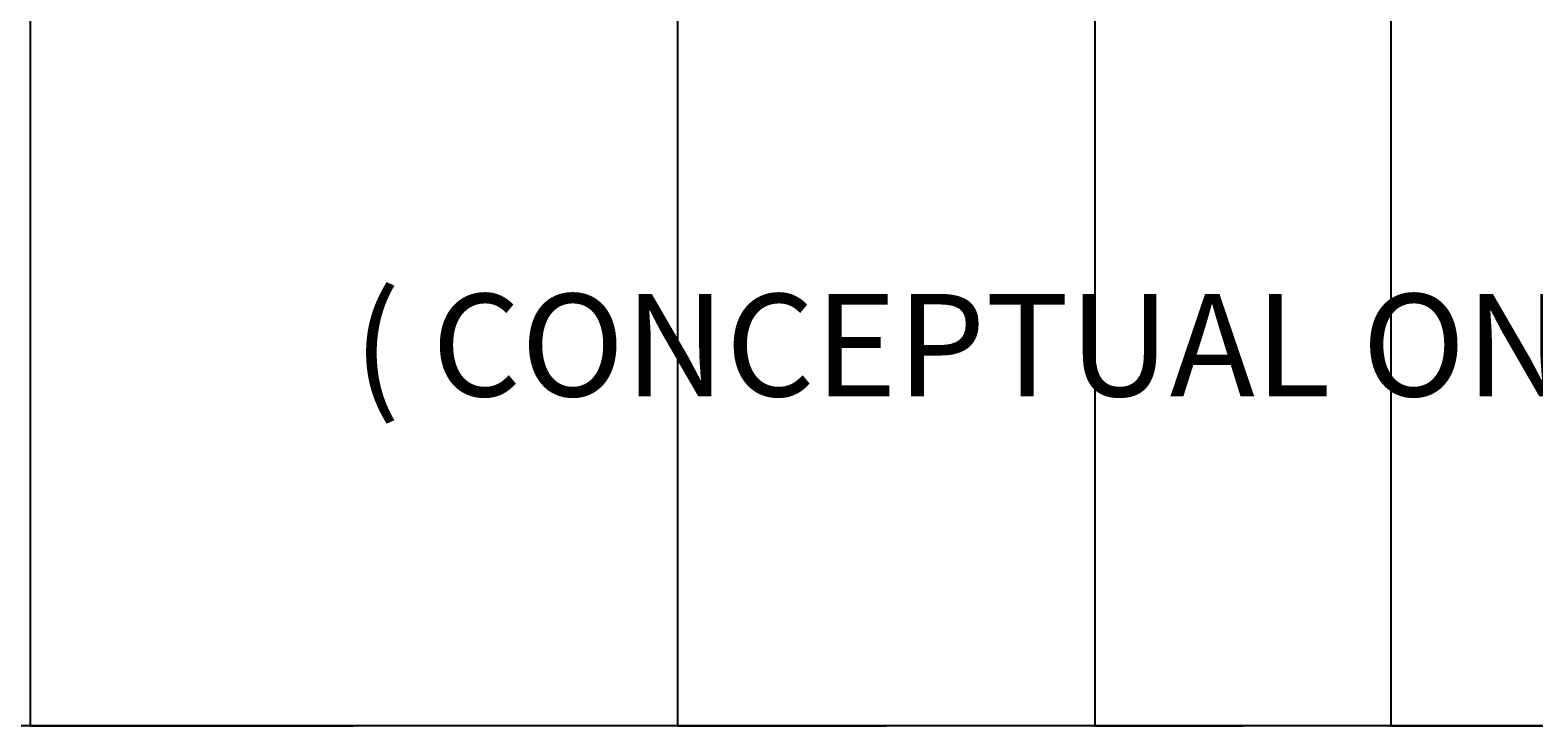
# Model space of a CAD drawing. Units: inches. Extents: x -32109 to 33221, y -19197 to 7608.
# Tile 4 of 25: x -6953 to -741, y -19197 to -16323. Entities that reach past the tile are written whole.
import ezdxf

# ---------------------------------------------------------------- set-up
doc = ezdxf.new("R2010")
doc.units = ezdxf.units.IN
doc.header["$MEASUREMENT"] = 0
doc.layers.add('A-ANNO-DIMS', color=2, linetype='Continuous', lineweight=18)
doc.layers.add('A-ANNO-TEXT', color=7, linetype='Continuous', lineweight=25)
doc.styles.get("Standard").update_dxf_attribs({"font": 'arial.ttf'})
doc.dimstyles.get("Standard").update_dxf_attribs({"dimtxt": 0.18, "dimasz": 0.18, "dimexe": 0.18, "dimexo": 0.0625, "dimgap": 0.09, "dimtad": 0, "dimtih": 1, "dimtoh": 1, "dimdec": 4, "dimzin": 0, "dimdsep": 46, "dimtxsty": 'Standard', "dimcen": 0.09, "dimadec": 0, "dimazin": 0, "dimtfac": 1, "dimtdec": 4, "dimtofl": 0, "dimtmove": 0, "dimatfit": 3, "dimfxl": 1, "dimtolj": 1, "dimtzin": 0, "dimarcsym": 0})

# ---------------------------------------------------------------- blocks, each defined once
blk = doc.blocks.new('*D13')
at = {"layer": 'A-ANNO-DIMS', "color": 0, "lineweight": -2, "transparency": 16777216}
for p, q in [((-21916.3, -16214.9), (-21916.3, -19197.3)), ((5067.2, -16244.2), (5067.2, -19197.3)), ((-21916.1, -19197.2), (-8425, -19197.2)), ((5067, -19197.2), (-8424.2, -19197.2))]:
    blk.add_line(p, q, dxfattribs=at)
at = {"layer": 'A-ANNO-DIMS', "color": 0, "transparency": 16777216}
for points in [[(-21916.1, -19197.1), (-21916.1, -19197.2), (-21916.3, -19197.2)], [(5067, -19197.1), (5067, -19197.2), (5067.2, -19197.2)]]:
    blk.add_solid(points, dxfattribs=at)
at = {"layer": 'Defpoints', "color": 0, "transparency": 16777216}
for p in [(-21916.3, -16214.8), (5067.2, -16244.1), (5067.2, -19197.2)]:
    blk.add_point(p, dxfattribs=at)
at = {"layer": 'A-ANNO-DIMS', "color": 0, "transparency": 16777216, "insert": (-8424.6, -19197.2), "char_height": 0.18, "attachment_point": 5}
blk.add_mtext('\\A1;26983', dxfattribs=at)
blk = doc.blocks.new('*D15')
at = {"layer": 'A-ANNO-DIMS', "color": 0, "lineweight": -2, "transparency": 16777216}
for p, q in [((-8664.1, -16214.9), (-8664.1, -19197.3)), ((-6952.8, -16214.9), (-6952.8, -19197.3)), ((-8664, -19197.2), (-7808.9, -19197.2)), ((-6953, -19197.2), (-7808, -19197.2))]:
    blk.add_line(p, q, dxfattribs=at)
at = {"layer": 'A-ANNO-DIMS', "color": 0, "transparency": 16777216}
for points in [[(-8664, -19197.1), (-8664, -19197.2), (-8664.1, -19197.2)], [(-6953, -19197.1), (-6953, -19197.2), (-6952.8, -19197.2)]]:
    blk.add_solid(points, dxfattribs=at)
at = {"layer": 'Defpoints', "color": 0, "transparency": 16777216}
for p in [(-8664.1, -16214.8), (-6952.8, -16214.8), (-6952.8, -19197.2)]:
    blk.add_point(p, dxfattribs=at)
at = {"layer": 'A-ANNO-DIMS', "color": 0, "transparency": 16777216, "insert": (-7808.5, -19197.2), "char_height": 0.18, "attachment_point": 5}
blk.add_mtext('\\A1;1711.4', dxfattribs=at)
blk = doc.blocks.new('*D103')
at = {"layer": 'A-ANNO-DIMS', "color": 0, "lineweight": -2, "transparency": 16777216}
for p, q in [((-6952.8, -16214.9), (-6952.8, -19197.3)), ((-4279, -16214.9), (-4279, -19197.3)), ((-6952.6, -19197.2), (-5616.2, -19197.2)), ((-4279.1, -19197.2), (-5615.5, -19197.2))]:
    blk.add_line(p, q, dxfattribs=at)
at = {"layer": 'A-ANNO-DIMS', "color": 0, "transparency": 16777216}
for points in [[(-6952.6, -19197.1), (-6952.6, -19197.2), (-6952.8, -19197.2)], [(-4279.1, -19197.1), (-4279.1, -19197.2), (-4279, -19197.2)]]:
    blk.add_solid(points, dxfattribs=at)
at = {"layer": 'Defpoints', "color": 0, "transparency": 16777216}
for p in [(-6952.8, -16214.8), (-4279, -16214.8), (-4279, -19197.2)]:
    blk.add_point(p, dxfattribs=at)
at = {"layer": 'A-ANNO-DIMS', "color": 0, "transparency": 16777216, "insert": (-5615.9, -19197.2), "char_height": 0.18, "attachment_point": 5}
blk.add_mtext('\\A1;2674', dxfattribs=at)
blk = doc.blocks.new('*D104')
at = {"layer": 'A-ANNO-DIMS', "color": 0, "lineweight": -2, "transparency": 16777216}
for p, q in [((-4279, -16214.9), (-4279, -19197.3)), ((-2554.3, -16214.9), (-2554.3, -19197.3)), ((-4278.8, -19197.2), (-3417.1, -19197.2)), ((-2554.5, -19197.2), (-3416.2, -19197.2))]:
    blk.add_line(p, q, dxfattribs=at)
at = {"layer": 'A-ANNO-DIMS', "color": 0, "transparency": 16777216}
for points in [[(-4278.8, -19197.1), (-4278.8, -19197.2), (-4279, -19197.2)], [(-2554.5, -19197.1), (-2554.5, -19197.2), (-2554.3, -19197.2)]]:
    blk.add_solid(points, dxfattribs=at)
at = {"layer": 'Defpoints', "color": 0, "transparency": 16777216}
for p in [(-4279, -16214.8), (-2554.3, -16214.8), (-2554.3, -19197.2)]:
    blk.add_point(p, dxfattribs=at)
at = {"layer": 'A-ANNO-DIMS', "color": 0, "transparency": 16777216, "insert": (-3416.6, -19197.2), "char_height": 0.18, "attachment_point": 5}
blk.add_mtext('\\A1;1724.6', dxfattribs=at)
blk = doc.blocks.new('*D105')
at = {"layer": 'A-ANNO-DIMS', "color": 0, "lineweight": -2, "transparency": 16777216}
for p, q in [((-2554.3, -16214.9), (-2554.3, -19197.3)), ((-1331.3, -16214.9), (-1331.3, -19197.3)), ((-2554.1, -19197.2), (-1943.2, -19197.2)), ((-1331.5, -19197.2), (-1942.5, -19197.2))]:
    blk.add_line(p, q, dxfattribs=at)
at = {"layer": 'A-ANNO-DIMS', "color": 0, "transparency": 16777216}
for points in [[(-2554.1, -19197.1), (-2554.1, -19197.2), (-2554.3, -19197.2)], [(-1331.5, -19197.1), (-1331.5, -19197.2), (-1331.3, -19197.2)]]:
    blk.add_solid(points, dxfattribs=at)
at = {"layer": 'Defpoints', "color": 0, "transparency": 16777216}
for p in [(-2554.3, -16214.8), (-1331.3, -16214.8), (-1331.3, -19197.2)]:
    blk.add_point(p, dxfattribs=at)
at = {"layer": 'A-ANNO-DIMS', "color": 0, "transparency": 16777216, "insert": (-1942.8, -19197.2), "char_height": 0.18, "attachment_point": 5}
blk.add_mtext('\\A1;1223', dxfattribs=at)
blk = doc.blocks.new('*D106')
at = {"layer": 'A-ANNO-DIMS', "color": 0, "lineweight": -2, "transparency": 16777216}
for p, q in [((-1331.3, -16214.9), (-1331.3, -19197.3)), ((2144.2, -16214.9), (2144.2, -19197.3)), ((-1331.1, -19197.2), (406, -19197.2)), ((2144.1, -19197.2), (406.9, -19197.2))]:
    blk.add_line(p, q, dxfattribs=at)
at = {"layer": 'A-ANNO-DIMS', "color": 0, "transparency": 16777216}
for points in [[(-1331.1, -19197.1), (-1331.1, -19197.2), (-1331.3, -19197.2)], [(2144.1, -19197.1), (2144.1, -19197.2), (2144.2, -19197.2)]]:
    blk.add_solid(points, dxfattribs=at)
at = {"layer": 'Defpoints', "color": 0, "transparency": 16777216}
for p in [(-1331.3, -16214.8), (2144.2, -16214.8), (2144.2, -19197.2)]:
    blk.add_point(p, dxfattribs=at)
at = {"layer": 'A-ANNO-DIMS', "color": 0, "transparency": 16777216, "insert": (406.5, -19197.2), "char_height": 0.18, "attachment_point": 5}
blk.add_mtext('\\A1;3475.6', dxfattribs=at)

msp = doc.modelspace()

# ---------------------------------------------------------------- texts
at = {"layer": 'A-ANNO-TEXT'}
msp.add_text('  ( CONCEPTUAL ONLY   NO DIMENSIONS )', height=423.03854, dxfattribs=at).set_placement((-5876.467, -17835.723))

# ---------------------------------------------------------------- dimensions: what is measured, and where the dimension line sits
at = {"layer": 'A-ANNO-DIMS'}
for base, p1, p2, override, picture, middle in [((5067.151, -19197.169), (-21916.328, -16214.811), (5067.151, -16244.113), {"dimdec": 0, "dimlfac": 1, "dimrnd": 0, "dimzin": 0, "dimdsep": 46, "dimlunit": 2}, '*D13', (-8424.588, -19197.169)), ((-6952.774, -19197.169), (-8664.143, -16214.811), (-6952.774, -16214.811), {"dimdec": 1, "dimlfac": 1, "dimrnd": 0, "dimzin": 0, "dimdsep": 46, "dimlunit": 2}, '*D15', (-7808.458, -19197.169)), ((-4278.952, -19197.169), (-6952.774, -16214.811), (-4278.952, -16214.811), {"dimdec": 0, "dimlfac": 1, "dimrnd": 0, "dimzin": 0, "dimdsep": 46, "dimlunit": 2}, '*D103', (-5615.863, -19197.169)), ((-2554.321, -19197.169), (-4278.952, -16214.811), (-2554.321, -16214.811), {"dimdec": 1, "dimlfac": 1, "dimrnd": 0, "dimzin": 0, "dimdsep": 46, "dimlunit": 2}, '*D104', (-3416.636, -19197.169)), ((-1331.314, -19197.169), (-2554.321, -16214.811), (-1331.314, -16214.811), {"dimdec": 0, "dimlfac": 1, "dimrnd": 0, "dimzin": 0, "dimdsep": 46, "dimlunit": 2}, '*D105', (-1942.818, -19197.169)), ((2144.248, -19197.169), (-1331.314, -16214.811), (2144.248, -16214.811), {"dimdec": 1, "dimlfac": 1, "dimrnd": 0, "dimzin": 0, "dimdsep": 46, "dimlunit": 2}, '*D106', (406.467, -19197.169))]:
    dim = msp.add_linear_dim(base=base, p1=p1, p2=p2, dimstyle='Standard', override=override, dxfattribs=at)
    dim.commit()
    dim.dimension.update_dxf_attribs({"geometry": picture, "text_midpoint": middle})

doc.saveas('drawing.dxf')
